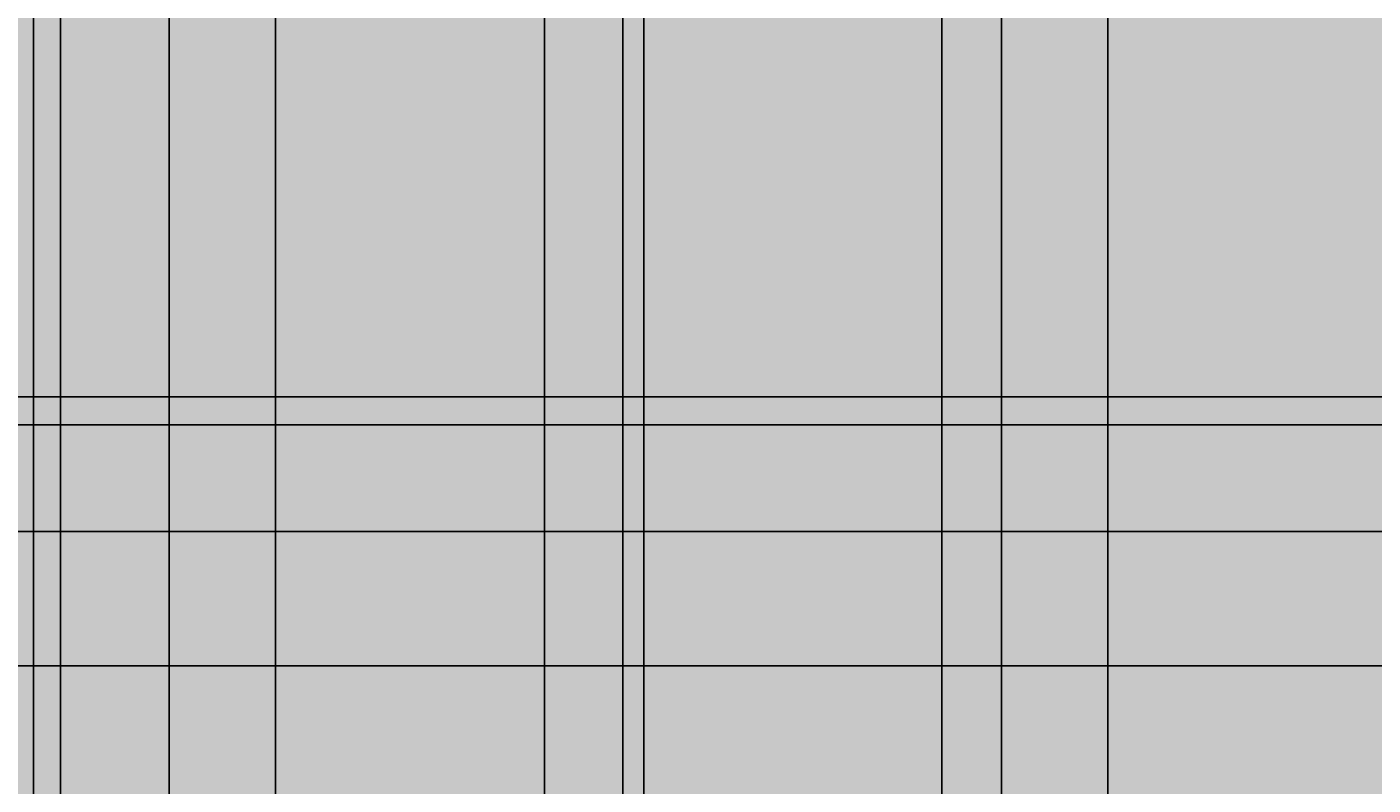
# Model space of a CAD drawing. Units: inches. Extents: x 818 to 1898, y 976 to 2364.
# Tile 86 of 96: x 1439 to 1539, y 2054 to 2111. Entities that reach past the tile are written whole.
import ezdxf

# ---------------------------------------------------------------- set-up
doc = ezdxf.new("R2010")
doc.units = ezdxf.units.IN
doc.header["$LTSCALE"] = 5
doc.header["$MEASUREMENT"] = 0
doc.layers.add('A-ANNO-DIMS', color=2, linetype='Continuous', lineweight=18)
doc.layers.add('L-PLNT-PATT', color=114, linetype='Continuous', lineweight=9, true_color=0x139b48)
doc.styles.get("Standard").update_dxf_attribs({"font": 'arial.ttf'})
doc.dimstyles.get("Standard").update_dxf_attribs({"dimtxt": 0.18, "dimasz": 0.18, "dimexe": 0.18, "dimexo": 0.0625, "dimgap": 0.09, "dimtad": 0, "dimtih": 1, "dimtoh": 1, "dimdec": 4, "dimzin": 0, "dimdsep": 46, "dimtxsty": 'Standard', "dimcen": 0.09, "dimadec": 0, "dimazin": 0, "dimtfac": 1, "dimtdec": 4, "dimtofl": 0, "dimtmove": 0, "dimatfit": 3, "dimfxl": 1, "dimtolj": 1, "dimtzin": 0, "dimarcsym": 0})

# ---------------------------------------------------------------- blocks, each defined once
blk = doc.blocks.new('*D86')
at = {"layer": 'A-ANNO-DIMS', "color": 0, "lineweight": -2, "ltscale": 5, "transparency": 16777216}
for p, q in [((1258.73, 2053.14), (1258.73, 2363.87)), ((1258.91, 2363.69), (1486.43, 2363.69)), ((1714.55, 2363.69), (1487.02, 2363.69)), ((1714.73, 2053.14), (1714.73, 2363.87))]:
    blk.add_line(p, q, dxfattribs=at)
at = {"layer": 'A-ANNO-DIMS', "color": 0, "ltscale": 5, "transparency": 16777216}
for points in [[(1258.91, 2363.72), (1258.91, 2363.66), (1258.73, 2363.69)], [(1714.55, 2363.72), (1714.55, 2363.66), (1714.73, 2363.69)]]:
    blk.add_solid(points, dxfattribs=at)
at = {"layer": 'Defpoints', "color": 0, "ltscale": 5, "transparency": 16777216}
for p in [(1714.73, 2363.69), (1258.73, 2053.08), (1714.73, 2053.08)]:
    blk.add_point(p, dxfattribs=at)
at = {"layer": 'A-ANNO-DIMS', "color": 0, "ltscale": 5, "transparency": 16777216, "insert": (1486.73, 2363.69), "char_height": 0.18, "attachment_point": 5}
blk.add_mtext('\\A1;456', dxfattribs=at)
blk = doc.blocks.new('*D99')
at = {"layer": 'A-ANNO-DIMS', "color": 0, "lineweight": -2, "ltscale": 5, "transparency": 16777216}
for p, q in [((1391.88, 1071.12), (1391.88, 2363.87)), ((1392.06, 2363.69), (1420.45, 2363.69)), ((1449.64, 2363.69), (1421.24, 2363.69)), ((1449.82, 1071.12), (1449.82, 2363.87))]:
    blk.add_line(p, q, dxfattribs=at)
at = {"layer": 'A-ANNO-DIMS', "color": 0, "ltscale": 5, "transparency": 16777216}
for points in [[(1392.06, 2363.72), (1392.06, 2363.66), (1391.88, 2363.69)], [(1449.64, 2363.72), (1449.64, 2363.66), (1449.82, 2363.69)]]:
    blk.add_solid(points, dxfattribs=at)
at = {"layer": 'Defpoints', "color": 0, "ltscale": 5, "transparency": 16777216}
for p in [(1449.82, 2363.69), (1391.88, 1071.06), (1449.82, 1071.06)]:
    blk.add_point(p, dxfattribs=at)
at = {"layer": 'A-ANNO-DIMS', "color": 0, "ltscale": 5, "transparency": 16777216, "insert": (1420.85, 2363.69), "char_height": 0.18, "attachment_point": 5}
blk.add_mtext('\\A1;57.94', dxfattribs=at)
blk = doc.blocks.new('*D100')
at = {"layer": 'A-ANNO-DIMS', "color": 0, "lineweight": -2, "ltscale": 5, "transparency": 16777216}
for p, q in [((1449.82, 1071.12), (1449.82, 2363.87)), ((1450, 2363.69), (1478.17, 2363.69)), ((1507.12, 2363.69), (1478.95, 2363.69)), ((1507.3, 1071.12), (1507.3, 2363.87))]:
    blk.add_line(p, q, dxfattribs=at)
at = {"layer": 'A-ANNO-DIMS', "color": 0, "ltscale": 5, "transparency": 16777216}
for points in [[(1450, 2363.72), (1450, 2363.66), (1449.82, 2363.69)], [(1507.12, 2363.72), (1507.12, 2363.66), (1507.3, 2363.69)]]:
    blk.add_solid(points, dxfattribs=at)
at = {"layer": 'Defpoints', "color": 0, "ltscale": 5, "transparency": 16777216}
for p in [(1507.3, 2363.69), (1449.82, 1071.06), (1507.3, 1071.06)]:
    blk.add_point(p, dxfattribs=at)
at = {"layer": 'A-ANNO-DIMS', "color": 0, "ltscale": 5, "transparency": 16777216, "insert": (1478.56, 2363.69), "char_height": 0.18, "attachment_point": 5}
blk.add_mtext('\\A1;57.48', dxfattribs=at)
blk = doc.blocks.new('*D101')
at = {"layer": 'A-ANNO-DIMS', "color": 0, "lineweight": -2, "ltscale": 5, "transparency": 16777216}
for p, q in [((1507.3, 1071.12), (1507.3, 2363.87)), ((1507.48, 2363.69), (1536, 2363.69)), ((1565.3, 2363.69), (1536.78, 2363.69)), ((1565.48, 1071.12), (1565.48, 2363.87))]:
    blk.add_line(p, q, dxfattribs=at)
at = {"layer": 'A-ANNO-DIMS', "color": 0, "ltscale": 5, "transparency": 16777216}
for points in [[(1507.48, 2363.72), (1507.48, 2363.66), (1507.3, 2363.69)], [(1565.3, 2363.72), (1565.3, 2363.66), (1565.48, 2363.69)]]:
    blk.add_solid(points, dxfattribs=at)
at = {"layer": 'Defpoints', "color": 0, "ltscale": 5, "transparency": 16777216}
for p in [(1565.48, 2363.69), (1507.3, 1071.06), (1565.48, 1071.06)]:
    blk.add_point(p, dxfattribs=at)
at = {"layer": 'A-ANNO-DIMS', "color": 0, "ltscale": 5, "transparency": 16777216, "insert": (1536.39, 2363.69), "char_height": 0.18, "attachment_point": 5}
blk.add_mtext('\\A1;58.19', dxfattribs=at)
blk = doc.blocks.new('*D141')
at = {"layer": 'A-ANNO-DIMS', "color": 0, "lineweight": -2, "ltscale": 5, "transparency": 16777216}
for p, q in [((1218.17, 2083.26), (1897.92, 2083.26)), ((1897.74, 2083.08), (1897.74, 2073.44)), ((1897.74, 2063.44), (1897.74, 2073.08)), ((1198.17, 2063.26), (1897.92, 2063.26))]:
    blk.add_line(p, q, dxfattribs=at)
at = {"layer": 'A-ANNO-DIMS', "color": 0, "ltscale": 5, "transparency": 16777216}
for points in [[(1897.71, 2083.08), (1897.77, 2083.08), (1897.74, 2083.26)], [(1897.71, 2063.44), (1897.77, 2063.44), (1897.74, 2063.26)]]:
    blk.add_solid(points, dxfattribs=at)
at = {"layer": 'Defpoints', "color": 0, "ltscale": 5, "transparency": 16777216}
for p in [(1218.11, 2083.26), (1198.11, 2063.26), (1897.74, 2063.26)]:
    blk.add_point(p, dxfattribs=at)
at = {"layer": 'A-ANNO-DIMS', "color": 0, "ltscale": 5, "transparency": 16777216, "insert": (1897.74, 2073.26), "char_height": 0.18, "attachment_point": 5}
blk.add_mtext('\\A1;20', dxfattribs=at)
blk = doc.blocks.new('*D142')
at = {"layer": 'A-ANNO-DIMS', "color": 0, "lineweight": -2, "ltscale": 5, "transparency": 16777216}
for p, q in [((1208.17, 2073.26), (1897.92, 2073.26)), ((1897.74, 2073.08), (1897.74, 2068.44)), ((1897.74, 2063.44), (1897.74, 2068.08)), ((1198.17, 2063.26), (1897.92, 2063.26))]:
    blk.add_line(p, q, dxfattribs=at)
at = {"layer": 'A-ANNO-DIMS', "color": 0, "ltscale": 5, "transparency": 16777216}
for points in [[(1897.71, 2073.08), (1897.77, 2073.08), (1897.74, 2073.26)], [(1897.71, 2063.44), (1897.77, 2063.44), (1897.74, 2063.26)]]:
    blk.add_solid(points, dxfattribs=at)
at = {"layer": 'Defpoints', "color": 0, "ltscale": 5, "transparency": 16777216}
for p in [(1208.11, 2073.26), (1897.74, 2073.26), (1198.11, 2063.26)]:
    blk.add_point(p, dxfattribs=at)
at = {"layer": 'A-ANNO-DIMS', "color": 0, "ltscale": 5, "transparency": 16777216, "insert": (1897.74, 2068.26), "char_height": 0.18, "attachment_point": 5}
blk.add_mtext('\\A1;10', dxfattribs=at)
blk = doc.blocks.new('*D161')
at = {"layer": 'A-ANNO-DIMS', "color": 0, "lineweight": -2, "ltscale": 5, "transparency": 16777216}
for p, q in [((1429.23, 1876.14), (1429.23, 2363.87)), ((1429.41, 2363.69), (1509.59, 2363.69)), ((1590.55, 2363.69), (1510.36, 2363.69)), ((1590.73, 1876.14), (1590.73, 2363.87))]:
    blk.add_line(p, q, dxfattribs=at)
at = {"layer": 'A-ANNO-DIMS', "color": 0, "ltscale": 5, "transparency": 16777216}
for points in [[(1429.41, 2363.72), (1429.41, 2363.66), (1429.23, 2363.69)], [(1590.55, 2363.72), (1590.55, 2363.66), (1590.73, 2363.69)]]:
    blk.add_solid(points, dxfattribs=at)
at = {"layer": 'Defpoints', "color": 0, "ltscale": 5, "transparency": 16777216}
for p in [(1590.73, 2363.69), (1429.23, 1876.08), (1590.73, 1876.08)]:
    blk.add_point(p, dxfattribs=at)
at = {"layer": 'A-ANNO-DIMS', "color": 0, "ltscale": 5, "transparency": 16777216, "insert": (1509.98, 2363.69), "char_height": 0.18, "attachment_point": 5}
blk.add_mtext('\\A1;161.5', dxfattribs=at)
blk = doc.blocks.new('*D169')
at = {"layer": 'A-ANNO-DIMS', "color": 0, "lineweight": -2, "ltscale": 5, "transparency": 16777216}
for p, q in [((1441.73, 1600.14), (1441.73, 2363.87)), ((1441.91, 2363.69), (1459.51, 2363.69)), ((1477.55, 2363.69), (1459.94, 2363.69)), ((1477.73, 1600.14), (1477.73, 2363.87))]:
    blk.add_line(p, q, dxfattribs=at)
at = {"layer": 'A-ANNO-DIMS', "color": 0, "ltscale": 5, "transparency": 16777216}
for points in [[(1441.91, 2363.72), (1441.91, 2363.66), (1441.73, 2363.69)], [(1477.55, 2363.72), (1477.55, 2363.66), (1477.73, 2363.69)]]:
    blk.add_solid(points, dxfattribs=at)
at = {"layer": 'Defpoints', "color": 0, "ltscale": 5, "transparency": 16777216}
for p in [(1477.73, 2363.69), (1441.73, 1600.08), (1477.73, 1600.08)]:
    blk.add_point(p, dxfattribs=at)
at = {"layer": 'A-ANNO-DIMS', "color": 0, "ltscale": 5, "transparency": 16777216, "insert": (1459.73, 2363.69), "char_height": 0.18, "attachment_point": 5}
blk.add_mtext('\\A1;36', dxfattribs=at)
blk = doc.blocks.new('*D196')
at = {"layer": 'A-ANNO-DIMS', "color": 0, "lineweight": -2, "ltscale": 5, "transparency": 16777216}
for p, q in [((1439.73, 1526.73), (1439.73, 2363.87)), ((1439.91, 2363.69), (1448.51, 2363.69)), ((1457.55, 2363.69), (1448.94, 2363.69)), ((1457.73, 1526.73), (1457.73, 2363.87))]:
    blk.add_line(p, q, dxfattribs=at)
at = {"layer": 'A-ANNO-DIMS', "color": 0, "ltscale": 5, "transparency": 16777216}
for points in [[(1439.91, 2363.72), (1439.91, 2363.66), (1439.73, 2363.69)], [(1457.55, 2363.72), (1457.55, 2363.66), (1457.73, 2363.69)]]:
    blk.add_solid(points, dxfattribs=at)
at = {"layer": 'Defpoints', "color": 0, "ltscale": 5, "transparency": 16777216}
for p in [(1457.73, 2363.69), (1439.73, 1526.67), (1457.73, 1526.67)]:
    blk.add_point(p, dxfattribs=at)
at = {"layer": 'A-ANNO-DIMS', "color": 0, "ltscale": 5, "transparency": 16777216, "insert": (1448.73, 2363.69), "char_height": 0.18, "attachment_point": 5}
blk.add_mtext('\\A1;18', dxfattribs=at)
blk = doc.blocks.new('*D238')
at = {"layer": 'A-ANNO-DIMS', "color": 0, "lineweight": -2, "ltscale": 5, "transparency": 16777216}
for p, q in [((1483.55, 1948.72), (1483.55, 2363.87)), ((1483.73, 2363.69), (1516.38, 2363.69)), ((1549.83, 2363.69), (1517.17, 2363.69)), ((1550.01, 1948.72), (1550.01, 2363.87))]:
    blk.add_line(p, q, dxfattribs=at)
at = {"layer": 'A-ANNO-DIMS', "color": 0, "ltscale": 5, "transparency": 16777216}
for points in [[(1483.73, 2363.72), (1483.73, 2363.66), (1483.55, 2363.69)], [(1549.83, 2363.72), (1549.83, 2363.66), (1550.01, 2363.69)]]:
    blk.add_solid(points, dxfattribs=at)
at = {"layer": 'Defpoints', "color": 0, "ltscale": 5, "transparency": 16777216}
for p in [(1550.01, 2363.69), (1483.55, 1948.66), (1550.01, 1948.66)]:
    blk.add_point(p, dxfattribs=at)
at = {"layer": 'A-ANNO-DIMS', "color": 0, "ltscale": 5, "transparency": 16777216, "insert": (1516.78, 2363.69), "char_height": 0.18, "attachment_point": 5}
blk.add_mtext('\\A1;66.47', dxfattribs=at)
blk = doc.blocks.new('*D244')
at = {"layer": 'A-ANNO-DIMS', "color": 0, "lineweight": -2, "ltscale": 5, "transparency": 16777216}
for p, q in [((1519.64, 1900.14), (1519.64, 2363.87)), ((1519.82, 2363.69), (1554.79, 2363.69)), ((1590.55, 2363.69), (1555.58, 2363.69)), ((1590.73, 1900.14), (1590.73, 2363.87))]:
    blk.add_line(p, q, dxfattribs=at)
at = {"layer": 'A-ANNO-DIMS', "color": 0, "ltscale": 5, "transparency": 16777216}
for points in [[(1519.82, 2363.72), (1519.82, 2363.66), (1519.64, 2363.69)], [(1590.55, 2363.72), (1590.55, 2363.66), (1590.73, 2363.69)]]:
    blk.add_solid(points, dxfattribs=at)
at = {"layer": 'Defpoints', "color": 0, "ltscale": 5, "transparency": 16777216}
for p in [(1590.73, 2363.69), (1519.64, 1900.08), (1590.73, 1900.08)]:
    blk.add_point(p, dxfattribs=at)
at = {"layer": 'A-ANNO-DIMS', "color": 0, "ltscale": 5, "transparency": 16777216, "insert": (1555.18, 2363.69), "char_height": 0.18, "attachment_point": 5}
blk.add_mtext('\\A1;71.08', dxfattribs=at)
blk = doc.blocks.new('*D258')
at = {"layer": 'A-ANNO-DIMS', "color": 0, "lineweight": -2, "ltscale": 5, "transparency": 16777216}
for p, q in [((1422.02, 2053.14), (1422.02, 2363.87)), ((1422.2, 2363.69), (1453.26, 2363.69)), ((1484.94, 2363.69), (1453.88, 2363.69)), ((1485.12, 2053.14), (1485.12, 2363.87))]:
    blk.add_line(p, q, dxfattribs=at)
at = {"layer": 'A-ANNO-DIMS', "color": 0, "ltscale": 5, "transparency": 16777216}
for points in [[(1422.2, 2363.72), (1422.2, 2363.66), (1422.02, 2363.69)], [(1484.94, 2363.72), (1484.94, 2363.66), (1485.12, 2363.69)]]:
    blk.add_solid(points, dxfattribs=at)
at = {"layer": 'Defpoints', "color": 0, "ltscale": 5, "transparency": 16777216}
for p in [(1485.12, 2363.69), (1422.02, 2053.08), (1485.12, 2053.08)]:
    blk.add_point(p, dxfattribs=at)
at = {"layer": 'A-ANNO-DIMS', "color": 0, "ltscale": 5, "transparency": 16777216, "insert": (1453.57, 2363.69), "char_height": 0.18, "attachment_point": 5}
blk.add_mtext('\\A1;63.1', dxfattribs=at)
blk = doc.blocks.new('*D281')
at = {"layer": 'A-ANNO-DIMS', "color": 0, "lineweight": -2, "ltscale": 5, "transparency": 16777216}
for p, q in [((1250.3, 1913.7), (1250.3, 2363.87)), ((1250.48, 2363.69), (1420.12, 2363.69)), ((1590.55, 2363.69), (1420.91, 2363.69)), ((1590.73, 2011.14), (1590.73, 2363.87))]:
    blk.add_line(p, q, dxfattribs=at)
at = {"layer": 'A-ANNO-DIMS', "color": 0, "ltscale": 5, "transparency": 16777216}
for points in [[(1250.48, 2363.72), (1250.48, 2363.66), (1250.3, 2363.69)], [(1590.55, 2363.72), (1590.55, 2363.66), (1590.73, 2363.69)]]:
    blk.add_solid(points, dxfattribs=at)
at = {"layer": 'Defpoints', "color": 0, "ltscale": 5, "transparency": 16777216}
for p in [(1590.73, 2363.69), (1590.73, 2011.08), (1250.3, 1913.64)]:
    blk.add_point(p, dxfattribs=at)
at = {"layer": 'A-ANNO-DIMS', "color": 0, "ltscale": 5, "transparency": 16777216, "insert": (1420.51, 2363.69), "char_height": 0.18, "attachment_point": 5}
blk.add_mtext('\\A1;340.4', dxfattribs=at)
blk = doc.blocks.new('*D282')
at = {"layer": 'A-ANNO-DIMS', "color": 0, "lineweight": -2, "ltscale": 5, "transparency": 16777216}
for p, q in [((1422.08, 2081.19), (1897.92, 2081.19)), ((1897.74, 2081.01), (1897.74, 1884.32)), ((1897.74, 1687.26), (1897.74, 1883.95)), ((1463.79, 1687.08), (1897.92, 1687.08))]:
    blk.add_line(p, q, dxfattribs=at)
at = {"layer": 'A-ANNO-DIMS', "color": 0, "ltscale": 5, "transparency": 16777216}
for points in [[(1897.71, 2081.01), (1897.77, 2081.01), (1897.74, 2081.19)], [(1897.71, 1687.26), (1897.77, 1687.26), (1897.74, 1687.08)]]:
    blk.add_solid(points, dxfattribs=at)
at = {"layer": 'Defpoints', "color": 0, "ltscale": 5, "transparency": 16777216}
for p in [(1422.02, 2081.19), (1897.74, 2081.19), (1463.73, 1687.08)]:
    blk.add_point(p, dxfattribs=at)
at = {"layer": 'A-ANNO-DIMS', "color": 0, "ltscale": 5, "transparency": 16777216, "insert": (1897.74, 1884.13), "char_height": 0.18, "attachment_point": 5}
blk.add_mtext('\\A1;394.1', dxfattribs=at)
blk = doc.blocks.new('*D288')
at = {"layer": 'A-ANNO-DIMS', "color": 0, "lineweight": -2, "ltscale": 5, "transparency": 16777216}
for p, q in [((1422.88, 1742.67), (1422.88, 2363.87)), ((1423.06, 2363.69), (1466.91, 2363.69)), ((1511.55, 2363.69), (1467.69, 2363.69)), ((1511.73, 1716.11), (1511.73, 2363.87))]:
    blk.add_line(p, q, dxfattribs=at)
at = {"layer": 'A-ANNO-DIMS', "color": 0, "ltscale": 5, "transparency": 16777216}
for points in [[(1423.06, 2363.72), (1423.06, 2363.66), (1422.88, 2363.69)], [(1511.55, 2363.72), (1511.55, 2363.66), (1511.73, 2363.69)]]:
    blk.add_solid(points, dxfattribs=at)
at = {"layer": 'Defpoints', "color": 0, "ltscale": 5, "transparency": 16777216}
for p in [(1511.73, 2363.69), (1422.88, 1742.61), (1511.73, 1716.05)]:
    blk.add_point(p, dxfattribs=at)
at = {"layer": 'A-ANNO-DIMS', "color": 0, "ltscale": 5, "transparency": 16777216, "insert": (1467.3, 2363.69), "char_height": 0.18, "attachment_point": 5}
blk.add_mtext('\\A1;88.85', dxfattribs=at)

msp = doc.modelspace()

# ---------------------------------------------------------------- hatches: boundary and pattern name
at = {"layer": 'L-PLNT-PATT', "ltscale": 5}
h = msp.add_hatch(color=256, dxfattribs=at)
h.dxf.hatch_style = 1
h.paths.add_polyline_path([(1789.7173, 2205.9709), (1083.7252, 2205.9709), (1083.7252, 2083.2623), (1218.1114, 2083.2623), (1218.1114, 2053.0782), (1390.6356, 2053.0782), (1390.6356, 2081.1881), (1399.6356, 2081.1881), (1413.02, 2081.1881), (1422.02, 2081.1881), (1422.02, 2053.0782), (1676.6446, 2053.0782), (1676.6446, 2081.1881), (1714.7251, 2081.1881), (1714.7251, 2081.6235), (1789.7173, 2081.6235)])
h.paths.add_polyline_path([(1388.6037, 2145.2461), (1388.6037, 2122.3767), (1373.4756, 2122.3767), (1373.4756, 2145.2461)], flags=16)
h.paths.add_polyline_path([(1408.6922, 2145.2461), (1423.8203, 2145.2461), (1423.8203, 2122.3767), (1408.6922, 2122.3767)], flags=16)
h.paths.add_polyline_path([(1353.3871, 2155.7839), (1353.3871, 2122.3767), (1338.259, 2122.3767), (1338.259, 2155.7839)], flags=16)
h.paths.add_polyline_path([(1443.9089, 2158.4222), (1459.037, 2158.4222), (1459.037, 2122.3767), (1443.9089, 2122.3767)], flags=16)
h.paths.add_polyline_path([(1318.1705, 2145.2461), (1318.1705, 2122.3767), (1303.0424, 2122.3767), (1303.0424, 2145.2461)], flags=16)
h.paths.add_polyline_path([(1479.1255, 2145.2461), (1494.2536, 2145.2461), (1494.2536, 2122.3767), (1479.1255, 2122.3767)], flags=16)
h.paths.add_polyline_path([(1282.9539, 2145.2461), (1282.9539, 2122.3767), (1267.8258, 2122.3767), (1267.8258, 2145.2461)], flags=16)
h.paths.add_polyline_path([(1514.3421, 2145.2461), (1529.4702, 2145.2461), (1529.4702, 2122.3767), (1514.3421, 2122.3767)], flags=16)
h.paths.add_polyline_path([(1247.7373, 2159.4296), (1247.7373, 2122.3767), (1232.6091, 2122.3767), (1232.6091, 2159.4296)], flags=16)
h.paths.add_polyline_path([(1549.5587, 2156.9246), (1564.6868, 2156.9246), (1564.6868, 2122.3767), (1549.5587, 2122.3767)], flags=16)
h.paths.add_polyline_path([(1212.5206, 2145.2461), (1212.5206, 2122.3767), (1197.3925, 2122.3767), (1197.3925, 2145.2461)], flags=16)
h.paths.add_polyline_path([(1584.7753, 2145.2461), (1599.9034, 2145.2461), (1599.9034, 2122.3767), (1584.7753, 2122.3767)], flags=16)
h.paths.add_polyline_path([(1185.1073, 2104.7786), (1190.6407, 2104.7786), (1185.1073, 2098.2505), (1179.5738, 2104.7786)], flags=16)
h.paths.add_polyline_path([(1619.9919, 2145.2461), (1635.1201, 2145.2461), (1635.1201, 2122.3767), (1619.9919, 2122.3767)], flags=16)
h.paths.add_polyline_path([(1655.2086, 2156.1761), (1670.3367, 2156.1761), (1670.3367, 2122.3767), (1655.2086, 2122.3767)], flags=16)
h.paths.add_polyline_path([(1686.5992, 2145.2461), (1701.7273, 2145.2461), (1701.7273, 2122.3767), (1686.5992, 2122.3767)], flags=16)
h.paths.add_polyline_path([(1715.7616, 2145.2461), (1730.8897, 2145.2461), (1730.8897, 2122.3767), (1715.7616, 2122.3767)], flags=16)
h.paths.add_polyline_path([(1753.1652, 2145.2461), (1776.3312, 2145.2461), (1776.3312, 2115.6891), (1753.1652, 2115.6891)], flags=16)
h.paths.add_polyline_path([(1191.4331, 2146.5159), (1176.7891, 2146.5159), (1176.7891, 2134.1516), (1191.4331, 2134.1516)], flags=24)

# ---------------------------------------------------------------- dimensions: what is measured, and where the dimension line sits
at = {"layer": 'A-ANNO-DIMS', "ltscale": 5}
for base, p1, p2, override, picture, middle in [((1590.7251, 2363.6929), (1250.3029, 1913.6401), (1590.7251, 2011.0782), {"dimdec": 1, "dimlfac": 1, "dimrnd": 0, "dimzin": 0, "dimdsep": 46, "dimlunit": 2}, '*D281', (1420.514, 2363.6929)), ((1714.7251, 2363.6929), (1258.7251, 2053.0782), (1714.7251, 2053.0782), {"dimdec": 0, "dimlfac": 1, "dimrnd": 0, "dimzin": 0, "dimdsep": 46, "dimlunit": 2}, '*D86', (1486.7251, 2363.6929)), ((1449.8196, 2363.6929), (1391.8757, 1071.0552), (1449.8196, 1071.0552), {"dimdec": 2, "dimlfac": 1, "dimrnd": 0, "dimzin": 0, "dimdsep": 46, "dimlunit": 2}, '*D99', (1420.8477, 2363.6929)), ((1485.1216, 2363.6929), (1422.02, 2053.0782), (1485.1216, 2053.0782), {"dimdec": 1, "dimlfac": 1, "dimrnd": 0, "dimzin": 0, "dimdsep": 46, "dimlunit": 2}, '*D258', (1453.5708, 2363.6929)), ((1511.7251, 2363.6929), (1422.8756, 1742.6113), (1511.7251, 1716.0454), {"dimdec": 2, "dimlfac": 1, "dimrnd": 0, "dimzin": 0, "dimdsep": 46, "dimlunit": 2}, '*D288', (1467.3004, 2363.6929)), ((1590.7251, 2363.6929), (1429.2251, 1876.0782), (1590.7251, 1876.0782), {"dimdec": 1, "dimlfac": 1, "dimrnd": 0, "dimzin": 0, "dimdsep": 46, "dimlunit": 2}, '*D161', (1509.9751, 2363.6929)), ((1457.7251, 2363.6929), (1439.7251, 1526.6712), (1457.7251, 1526.6712), {"dimdec": 0, "dimlfac": 1, "dimrnd": 0, "dimzin": 0, "dimdsep": 46, "dimlunit": 2}, '*D196', (1448.7251, 2363.6929)), ((1477.7251, 2363.6929), (1441.7251, 1600.0782), (1477.7251, 1600.0782), {"dimdec": 0, "dimlfac": 1, "dimrnd": 0, "dimzin": 0, "dimdsep": 46, "dimlunit": 2}, '*D169', (1459.7251, 2363.6929)), ((1507.2982, 2363.6929), (1449.8196, 1071.0552), (1507.2982, 1071.0552), {"dimdec": 2, "dimlfac": 1, "dimrnd": 0, "dimzin": 0, "dimdsep": 46, "dimlunit": 2}, '*D100', (1478.5589, 2363.6929)), ((1550.0109, 2363.6929), (1483.5451, 1948.6602), (1550.0109, 1948.6602), {"dimdec": 2, "dimlfac": 1, "dimrnd": 0, "dimzin": 0, "dimdsep": 46, "dimlunit": 2}, '*D238', (1516.778, 2363.6929)), ((1565.4835, 2363.6929), (1507.2982, 1071.0552), (1565.4835, 1071.0552), {"dimdec": 2, "dimlfac": 1, "dimrnd": 0, "dimzin": 0, "dimdsep": 46, "dimlunit": 2}, '*D101', (1536.3908, 2363.6929)), ((1590.7251, 2363.6929), (1519.6413, 1900.0782), (1590.7251, 1900.0782), {"dimdec": 2, "dimlfac": 1, "dimrnd": 0, "dimzin": 0, "dimdsep": 46, "dimlunit": 2}, '*D244', (1555.1832, 2363.6929))]:
    dim = msp.add_linear_dim(base=base, p1=p1, p2=p2, dimstyle='Standard', override=override, dxfattribs=at)
    dim.commit()
    dim.dimension.update_dxf_attribs({"geometry": picture, "text_midpoint": middle})
for base, p1, p2, override, picture, middle in [((1897.736, 2063.2623), (1218.1114, 2083.2623), (1198.1114, 2063.2623), {"dimdec": 0, "dimlfac": 1, "dimrnd": 0, "dimzin": 0, "dimdsep": 46, "dimlunit": 2}, '*D141', (1897.736, 2073.2623)), ((1897.736, 2081.1881), (1463.7251, 1687.0782), (1422.02, 2081.1881), {"dimdec": 1, "dimlfac": 1, "dimrnd": 0, "dimzin": 0, "dimdsep": 46, "dimlunit": 2}, '*D282', (1897.736, 1884.1332)), ((1897.736, 2073.2623), (1198.1114, 2063.2623), (1208.1114, 2073.2623), {"dimdec": 0, "dimlfac": 1, "dimrnd": 0, "dimzin": 0, "dimdsep": 46, "dimlunit": 2}, '*D142', (1897.736, 2068.2623))]:
    dim = msp.add_linear_dim(base=base, p1=p1, p2=p2, angle=90, dimstyle='Standard', override=override, dxfattribs=at)
    dim.commit()
    dim.dimension.update_dxf_attribs({"geometry": picture, "text_midpoint": middle})

doc.saveas('drawing.dxf')
